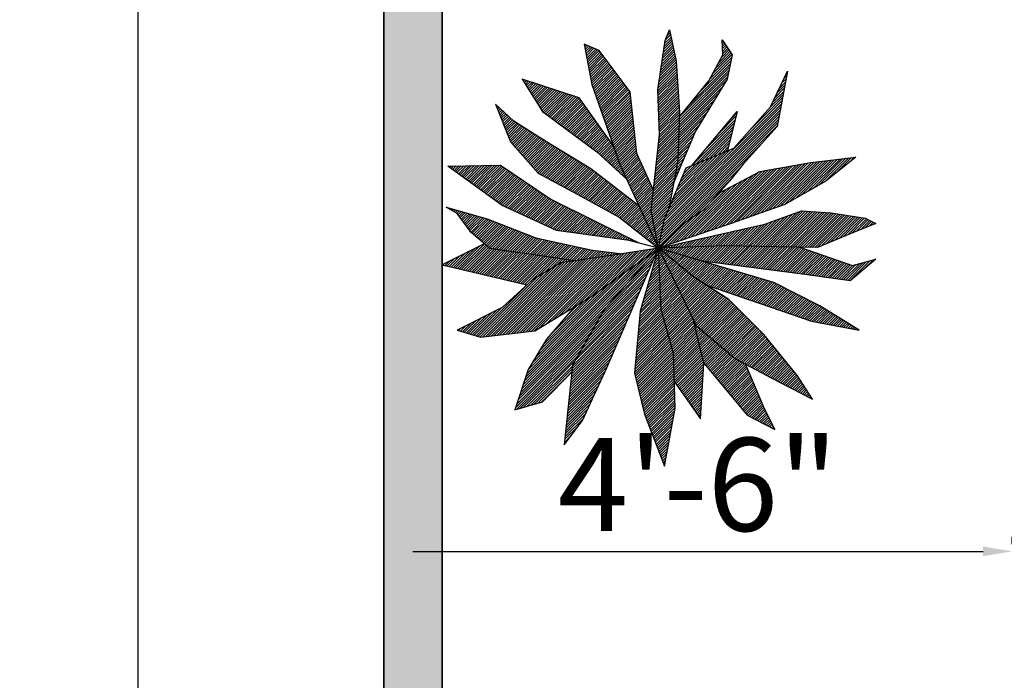
# Model space of a CAD drawing. Units: inches. Extents: x 3008 to 4088, y 1255 to 2137.
# Tile 11 of 30: x 3008 to 3093, y 1787 to 1844. Entities that reach past the tile are written whole.
import ezdxf

# ---------------------------------------------------------------- set-up
doc = ezdxf.new("R2010")
doc.units = ezdxf.units.IN
for name, color, linetype, lineweight in [('A-ANNO-DIMS', 2, 'Continuous', 18), ('C-PROP', 1, 'Continuous', 35), ('C-PROP-PATT', 9, 'Continuous', 13), ('L-PLNT', 3, 'Continuous', 13), ('vfolhas', 114, 'Continuous', 5)]:
    doc.layers.add(name, color=color, linetype=linetype, lineweight=lineweight)
for name, color, linetype in [('vfolha', 72, 'Continuous'), ('vfolha2', 110, 'Continuous'), ('vfolhas2', 102, 'Continuous')]:
    doc.layers.add(name, color=color, linetype=linetype)
doc.styles.get("Standard").update_dxf_attribs({"font": 'arial.ttf'})
doc.dimstyles.new('ISO-25', dxfattribs={"dimtxt": 8, "dimasz": 2.5, "dimexe": 1.25, "dimexo": 0.625, "dimtad": 1, "dimdec": 1, "dimlunit": 3, "dimtxsty": 'Standard', "dimcen": 2.5, "dimadec": 0, "dimazin": 0, "dimtfac": 1, "dimtdec": 1, "dimtmove": 0, "dimatfit": 3, "dimfxl": 1, "dimarcsym": 0})
pattern_1 = [(45, (-2446.5133113, 50.986076), (-0.004419417382, 0.004419417382), [])]

# ---------------------------------------------------------------- blocks, each defined once
blk = doc.blocks.new('*D2')
at = {"layer": 'A-ANNO-DIMS', "color": 0, "lineweight": -2, "transparency": 16777216}
for p, q in [((3039.041, 2003.966), (3017.26, 2003.966)), ((3018.51, 2001.466), (3018.51, 1346.466)), ((3039.041, 1343.966), (3017.26, 1343.966))]:
    blk.add_line(p, q, dxfattribs=at)
at = {"layer": 'A-ANNO-DIMS', "color": 0, "transparency": 16777216}
for points in [[(3018.093, 2001.466), (3018.927, 2001.466), (3018.51, 2003.966)], [(3018.093, 1346.466), (3018.927, 1346.466), (3018.51, 1343.966)]]:
    blk.add_solid(points, dxfattribs=at)
at = {"layer": 'Defpoints', "color": 0, "transparency": 16777216}
for p in [(3039.666, 2003.966), (3018.51, 1343.966), (3039.666, 1343.966)]:
    blk.add_point(p, dxfattribs=at)
at = {"layer": 'A-ANNO-DIMS', "color": 0, "transparency": 16777216, "insert": (3013.817, 1673.966), "char_height": 8, "attachment_point": 5, "rotation": 90}
blk.add_mtext("55'", dxfattribs=at)
blk = doc.blocks.new('*D3')
at = {"layer": 'A-ANNO-DIMS', "color": 0, "lineweight": -2, "transparency": 16777216}
for p, q in [((3039.666, 1798.574), (3039.666, 1799.199)), ((3093.666, 1798.574), (3093.666, 1799.199)), ((3042.166, 1797.949), (3091.166, 1797.949))]:
    blk.add_line(p, q, dxfattribs=at)
at = {"layer": 'A-ANNO-DIMS', "color": 0, "transparency": 16777216}
for points in [[(3042.166, 1798.366), (3042.166, 1797.532), (3039.666, 1797.949)], [(3091.166, 1798.366), (3091.166, 1797.532), (3093.666, 1797.949)]]:
    blk.add_solid(points, dxfattribs=at)
at = {"layer": 'Defpoints', "color": 0, "transparency": 16777216}
for p in [(3039.666, 1797.949), (3093.666, 1797.949), (3093.666, 1797.949)]:
    blk.add_point(p, dxfattribs=at)
at = {"layer": 'A-ANNO-DIMS', "color": 0, "transparency": 16777216, "insert": (3066.666, 1802.659), "char_height": 8, "attachment_point": 5}
blk.add_mtext('4\'-6"', dxfattribs=at)
blk = doc.blocks.new('arbusto_PB_verde_grande')
at = {"layer": 'vfolha2'}
h = blk.add_hatch(dxfattribs=at)
h.set_pattern_fill('ANSI31', color=256, scale=0.05, style=0)
h.set_pattern_definition(pattern_1)
h.paths.add_polyline_path([(0.0294, 0.3565), (0.0003, 0.0905), (0.0263, -0.0393), (0.047, 0.0623), (0.0619, 0.0973), (0.0937, 0.2657), (0.0996, 0.4347), (0.0879, 0.6131), (0.0645, 0.7227), (0.0499, 0.6851), (0.0236, 0.5129)])
h.paths.add_polyline_path([(0.3011, 0.4379), (0.1423, 0.2487), (0.2669, 0.3002)])
h.paths.add_polyline_path([(0.38, 0.2282), (0.237, 0.1519), (0.1843, 0.0936), (0.1112, 0.0436), (0.0263, -0.0393), (0.2806, 0.0467), (0.3683, 0.078), (0.4676, 0.1124), (0.6107, 0.1938), (0.7159, 0.2782), (0.5581, 0.2595)])
h.paths.add_polyline_path([(0.561, -0.2944), (0.7275, -0.3257), (0.5902, -0.2412), (0.4296, -0.1598), (0.0263, -0.0393), (0.1492, -0.1411), (0.1884, -0.166), (0.415, -0.2444)])
h.paths.add_polyline_path([(-0.2743, -0.4478), (-0.3035, -0.7263), (-0.2392, -0.6417), (-0.1546, -0.4572), (0.0263, -0.0393), (-0.1633, -0.2538)])
h.paths.add_polyline_path([(-0.5196, -0.2474), (-0.6774, -0.3257), (-0.5956, -0.3507), (-0.4057, -0.3288), (-0.2101, -0.21), (0.0263, -0.0393), (-0.1487, -0.0659), (-0.3152, -0.091), (-0.4145, -0.1505)])
h.paths.add_polyline_path([(-0.5255, 0.2501), (-0.7095, 0.247), (-0.5196, 0.1093), (-0.3298, 0.0217), (-0.0757, -0.0128), (-0.0423, -0.0215), (-0.3502, 0.1312)])
h = blk.add_hatch(dxfattribs=at)
h.set_pattern_fill('ANSI31', color=256, scale=0.05, style=0)
h.set_pattern_definition(pattern_1)
h.paths.add_polyline_path([(-0.1896, 0.297), (-0.0855, 0.2019), (-0.1078, 0.2501), (-0.132, 0.3187), (-0.251, 0.4848), (-0.4495, 0.5505), (-0.3795, 0.4379)])
h.paths.add_polyline_path([(0.0791, -0.4071), (0.0821, -0.5063), (0.1726, -0.6355), (0.1843, -0.4415), (0.149, -0.2918), (0.0263, -0.0393), (0.0353, -0.2538)])
at = {"layer": 'vfolhas'}
h = blk.add_hatch(dxfattribs=at)
h.set_pattern_fill('ANSI31', color=256, scale=0.05, style=0)
h.set_pattern_definition(pattern_1)
h.paths.add_polyline_path([(-0.0728, 0.5067), (-0.1808, 0.6506), (-0.2334, 0.6725), (-0.2071, 0.5318), (-0.1078, 0.2501), (0.0263, -0.0393), (0.0003, 0.0905), (0.0082, 0.1624), (-0.0494, 0.2908)])
h.paths.add_polyline_path([(0.099, 0.4193), (0.0937, 0.2657), (0.0791, 0.1881), (0.1551, 0.369), (0.2661, 0.5505), (0.2836, 0.635), (0.2485, 0.6882), (0.2514, 0.635), (0.2018, 0.5443)])
h.paths.add_polyline_path([(0.1229, 0.2407), (0.047, 0.0623), (0.0263, -0.0393), (0.1112, 0.0436), (0.1843, 0.0936), (0.2748, 0.1938), (0.3215, 0.2532), (0.4413, 0.3847), (0.4763, 0.5787), (0.4179, 0.4535), (0.2894, 0.3095)])
h.paths.add_polyline_path([(0.5815, -0.0378), (0.7071, 0.0154), (0.7859, 0.0467), (0.748, 0.0655), (0.6282, 0.0842), (0.526, 0.0905), (0.3974, 0.0436), (0.0263, -0.0393), (0.2573, -0.0315), (0.4383, -0.0347)])
h.paths.add_polyline_path([(0.5202, -0.0365), (0.4383, -0.0347), (0.2573, -0.0315), (0.0263, -0.0393), (0.1796, -0.0852), (0.5377, -0.1317), (0.6954, -0.1536), (0.7859, -0.0785), (0.7041, -0.1004)])
h.paths.add_polyline_path([(0.2719, -0.2193), (0.1492, -0.1411), (0.0263, -0.0393), (0.1579, -0.3101), (0.2952, -0.4258), (0.4179, -0.4916), (0.564, -0.5667), (0.5114, -0.4853), (0.3946, -0.3414)])
h.paths.add_polyline_path([(-0.0582, -0.4759), (-0.0231, -0.6198), (0.047, -0.8013), (0.0849, -0.5979), (0.0791, -0.4071), (0.0353, -0.2538), (0.0263, -0.0393), (-0.0377, -0.26)])
h.paths.add_polyline_path([(-0.2422, 0.1405), (-0.1107, 0.0686), (0.0263, -0.0393), (-0.0423, 0.1087), (-0.2101, 0.2376), (-0.3649, 0.3314), (-0.4787, 0.4034), (-0.543, 0.4629), (-0.4904, 0.3314), (-0.3941, 0.2219)])
h = blk.add_hatch(dxfattribs=at)
h.set_pattern_fill('ANSI31', color=256, scale=0.05, style=0)
h.set_pattern_definition(pattern_1)
h.paths.add_polyline_path([(-0.5722, 0.0623), (-0.7153, 0.103), (-0.6774, 0.0811), (-0.6277, 0.0154), (-0.5635, -0.041), (-0.2646, -0.0834), (-0.1487, -0.0659), (-0.1015, -0.0588), (-0.2042, -0.0472), (-0.4028, -0.0034)])
h.paths.add_polyline_path([(-0.5635, -0.041), (-0.5828, -0.024), (-0.7299, -0.0973), (-0.4334, -0.1679), (-0.4145, -0.1505), (-0.3152, -0.091), (-0.2646, -0.0834)])
h.paths.add_polyline_path([(-0.2769, -0.4727), (-0.2743, -0.4478), (-0.1633, -0.2538), (0.0263, -0.0393), (-0.2101, -0.21), (-0.2672, -0.2447), (-0.3649, -0.357), (-0.4291, -0.4634), (-0.4759, -0.6043), (-0.3795, -0.576)])
h = blk.add_hatch(dxfattribs=at)
h.set_pattern_fill('ANSI31', color=256, scale=0.05, style=0)
h.set_pattern_definition(pattern_1)
h.paths.add_polyline_path([(0.3361, -0.623), (0.4325, -0.6731), (0.3946, -0.5948), (0.3303, -0.4446), (0.2952, -0.4258), (0.1579, -0.3101), (0.149, -0.2918), (0.1843, -0.4415)])
at = {"layer": 'vfolha'}
for p, q in [((0.0263, -0.0393), (-0.1487, -0.0659)), ((0.0263, -0.0393), (-0.0377, -0.26)), ((0.0353, -0.2538), (0.0263, -0.0393)), ((0.5202, -0.0365), (0.7041, -0.1004)), ((0.5377, -0.1317), (0.1796, -0.0852)), ((0.7859, -0.0785), (0.6954, -0.1536)), ((0.7041, -0.1004), (0.7859, -0.0785)), ((0.6954, -0.1536), (0.5377, -0.1317)), ((0.3946, -0.3414), (0.2719, -0.2193)), ((-0.2672, -0.2447), (-0.3649, -0.357)), ((-0.0377, -0.26), (-0.0582, -0.4759)), ((0.0791, -0.4071), (0.0353, -0.2538)), ((0.1579, -0.3101), (0.2952, -0.4258)), ((0.5114, -0.4853), (0.3946, -0.3414)), ((0.0849, -0.5979), (0.0791, -0.4071)), ((0.2952, -0.4258), (0.4179, -0.4916)), ((0.4179, -0.4916), (0.564, -0.5667)), ((0.564, -0.5667), (0.5114, -0.4853)), ((0.047, -0.8013), (0.0849, -0.5979)), ((-0.0231, -0.6198), (0.047, -0.8013))]:
    blk.add_line(p, q, dxfattribs=at)
at = {"layer": 'vfolha2'}
for p, q in [((0.0499, 0.6851), (0.0645, 0.7227)), ((0.0645, 0.7227), (0.0879, 0.6131)), ((0.0236, 0.5129), (0.0499, 0.6851)), ((0.0879, 0.6131), (0.0996, 0.4347)), ((-0.4495, 0.5505), (-0.3795, 0.4379)), ((-0.251, 0.4848), (-0.4495, 0.5505)), ((-0.132, 0.3187), (-0.251, 0.4848)), ((0.0294, 0.3565), (0.0236, 0.5129)), ((-0.3795, 0.4379), (-0.1896, 0.297)), ((0.0996, 0.4347), (0.0937, 0.2657)), ((0.1434, 0.2501), (0.3011, 0.4379)), ((0.3011, 0.4379), (0.2661, 0.297)), ((0.0003, 0.0905), (0.0294, 0.3565)), ((-0.1896, 0.297), (-0.0822, 0.1989)), ((0.5581, 0.2595), (0.7159, 0.2782)), ((0.7159, 0.2782), (0.6107, 0.1938)), ((-0.7095, 0.247), (-0.5255, 0.2501)), ((-0.5196, 0.1093), (-0.7095, 0.247)), ((-0.5255, 0.2501), (-0.3502, 0.1312)), ((0.38, 0.2282), (0.5581, 0.2595)), ((0.237, 0.1519), (0.38, 0.2282)), ((0.6107, 0.1938), (0.4676, 0.1124)), ((-0.3298, 0.0217), (-0.5196, 0.1093)), ((-0.3502, 0.1312), (-0.0423, -0.0215)), ((0.0263, -0.0393), (0.0003, 0.0905)), ((0.3683, 0.078), (0.2806, 0.0467)), ((0.2806, 0.0467), (0.0263, -0.0393)), ((-0.0757, -0.0128), (-0.3298, 0.0217)), ((-0.1487, -0.0659), (-0.3152, -0.091)), ((-0.2101, -0.21), (0.0263, -0.0393)), ((0.0263, -0.0393), (-0.1633, -0.2538)), ((-0.1546, -0.4572), (0.0263, -0.0393)), ((0.4296, -0.1598), (0.0263, -0.0393)), ((0.0263, -0.0393), (0.1579, -0.3101)), ((-0.3152, -0.091), (-0.4145, -0.1505)), ((-0.4145, -0.1505), (-0.5196, -0.2474)), ((0.1884, -0.166), (0.415, -0.2444)), ((0.5902, -0.2412), (0.4296, -0.1598)), ((-0.4057, -0.3288), (-0.2101, -0.21)), ((-0.5196, -0.2474), (-0.6774, -0.3257)), ((-0.1633, -0.2538), (-0.2743, -0.4478)), ((0.415, -0.2444), (0.561, -0.2944)), ((0.7275, -0.3257), (0.5902, -0.2412)), ((0.1843, -0.4415), (0.149, -0.2918)), ((0.561, -0.2944), (0.7275, -0.3257)), ((-0.6774, -0.3257), (-0.5956, -0.3507)), ((-0.5956, -0.3507), (-0.4057, -0.3288)), ((0.1726, -0.6355), (0.1843, -0.4415)), ((-0.2743, -0.4478), (-0.3035, -0.7263)), ((0.0821, -0.5063), (0.1726, -0.6355)), ((-0.3035, -0.7263), (-0.2392, -0.6417))]:
    blk.add_line(p, q, dxfattribs=at)
at = {"layer": 'vfolhas2'}
for p, q in [((0.2514, 0.635), (0.2485, 0.6882)), ((0.2485, 0.6882), (0.2836, 0.635)), ((-0.2334, 0.6725), (-0.2071, 0.5318)), ((-0.1808, 0.6506), (-0.2334, 0.6725)), ((-0.0728, 0.5067), (-0.1808, 0.6506)), ((0.2018, 0.5443), (0.2514, 0.635)), ((0.2836, 0.635), (0.2661, 0.5505)), ((0.2661, 0.5505), (0.1551, 0.369)), ((0.4179, 0.4535), (0.4763, 0.5787)), ((0.4763, 0.5787), (0.4413, 0.3847)), ((-0.2071, 0.5318), (-0.1078, 0.2501)), ((0.099, 0.4193), (0.2018, 0.5443)), ((-0.0494, 0.2908), (-0.0728, 0.5067)), ((-0.543, 0.4629), (-0.4904, 0.3314)), ((-0.4787, 0.4034), (-0.543, 0.4629)), ((0.2894, 0.3095), (0.4179, 0.4535)), ((-0.3649, 0.3314), (-0.4787, 0.4034)), ((0.4413, 0.3847), (0.3215, 0.2532)), ((0.1551, 0.369), (0.078, 0.1855)), ((-0.4904, 0.3314), (-0.3941, 0.2219)), ((-0.2101, 0.2376), (-0.3649, 0.3314)), ((0.0082, 0.1624), (-0.0494, 0.2908)), ((0.1229, 0.2407), (0.2894, 0.3095)), ((-0.1078, 0.2501), (0.0263, -0.0393)), ((0.0937, 0.2657), (0.0619, 0.0973)), ((0.3215, 0.2532), (0.2748, 0.1938)), ((-0.3941, 0.2219), (-0.2422, 0.1405)), ((-0.0423, 0.1087), (-0.2101, 0.2376)), ((0.047, 0.0623), (0.1229, 0.2407)), ((0.2748, 0.1938), (0.1843, 0.0936)), ((-0.2422, 0.1405), (-0.1107, 0.0686)), ((0.4676, 0.1124), (0.3683, 0.078)), ((-0.6774, 0.0811), (-0.7153, 0.103)), ((-0.7153, 0.103), (-0.5722, 0.0623)), ((-0.6277, 0.0154), (-0.6774, 0.0811)), ((0.1843, 0.0936), (0.1112, 0.0436)), ((0.3974, 0.0436), (0.526, 0.0905)), ((0.526, 0.0905), (0.6282, 0.0842)), ((0.6282, 0.0842), (0.748, 0.0655)), ((-0.5722, 0.0623), (-0.4028, -0.0034)), ((-0.1107, 0.0686), (0.0263, -0.0393)), ((0.0263, -0.0393), (0.047, 0.0623)), ((0.0263, -0.0393), (0.3974, 0.0436)), ((0.1112, 0.0436), (0.0263, -0.0393)), ((0.7859, 0.0467), (0.7071, 0.0154)), ((0.748, 0.0655), (0.7859, 0.0467)), ((-0.5635, -0.041), (-0.6277, 0.0154)), ((0.7071, 0.0154), (0.5815, -0.0378)), ((-0.5828, -0.024), (-0.7299, -0.0973)), ((-0.4028, -0.0034), (-0.2042, -0.0472)), ((0.0263, -0.0393), (-0.0757, -0.0128)), ((0.2573, -0.0315), (0.0263, -0.0393)), ((0.4383, -0.0347), (0.2573, -0.0315)), ((-0.2646, -0.0834), (-0.5635, -0.041)), ((-0.2042, -0.0472), (-0.0983, -0.0591)), ((0.1492, -0.1411), (0.0263, -0.0393)), ((0.5815, -0.0378), (0.4383, -0.0347)), ((-0.7299, -0.0973), (-0.4334, -0.1679)), ((0.2719, -0.2193), (0.1492, -0.1411)), ((-0.3649, -0.357), (-0.4291, -0.4634)), ((0.1843, -0.4415), (0.3361, -0.623)), ((0.3946, -0.5948), (0.329, -0.4417)), ((-0.4291, -0.4634), (-0.4759, -0.6043)), ((-0.3795, -0.576), (-0.2769, -0.4727)), ((-0.2392, -0.6417), (-0.1546, -0.4572)), ((-0.0582, -0.4759), (-0.0231, -0.6198)), ((-0.4759, -0.6043), (-0.3795, -0.576)), ((0.4325, -0.6731), (0.3946, -0.5948)), ((0.3361, -0.623), (0.4325, -0.6731))]:
    blk.add_line(p, q, dxfattribs=at)

msp = doc.modelspace()

# ---------------------------------------------------------------- hatches: boundary and pattern name
at = {"layer": 'C-PROP-PATT'}
h = msp.add_hatch(color=256, dxfattribs=at)
h.dxf.hatch_style = 1
h.paths.add_polyline_path([(3519.666, 2003.966), (3039.666, 2003.966), (3039.666, 1343.966), (3051.666, 1343.966), (3051.666, 1348.966), (3044.666, 1348.966), (3044.666, 1998.966), (3514.666, 1998.966), (3514.666, 1348.966), (3219.666, 1348.966), (3219.666, 1343.966), (3519.666, 1343.966)])

# ---------------------------------------------------------------- linework, layer by layer
at = {"layer": 'C-PROP'}
for p, q in [((3039.666, 1343.966), (3039.666, 2003.966)), ((3044.666, 1348.966), (3044.666, 1998.966))]:
    msp.add_line(p, q, dxfattribs=at)

# ---------------------------------------------------------------- block references
at = {"layer": 'L-PLNT', "xscale": 24.60366729364114, "yscale": 24.60366729364114, "zscale": 24.60366729364114}
msp.add_blockref('arbusto_PB_verde_grande', (3062.624, 1824.969), dxfattribs=at)

# ---------------------------------------------------------------- dimensions: what is measured, and where the dimension line sits
at = {"layer": 'A-ANNO-DIMS'}
dim = msp.add_linear_dim(base=(3018.51, 1343.966), p1=(3039.666, 2003.966), p2=(3039.666, 1343.966), angle=90, dimstyle='ISO-25', override={"dimclrd": 0, "dimclre": 0, "dimclrt": 0}, dxfattribs=at)
dim.commit()
dim.dimension.update_dxf_attribs({"geometry": '*D2', "text_midpoint": (3013.817, 1673.966)})
dim = msp.add_linear_dim(base=(3093.666, 1797.949), p1=(3039.666, 1797.949), p2=(3093.666, 1797.949), dimstyle='ISO-25', override={"dimclrd": 0, "dimclre": 0, "dimclrt": 0}, dxfattribs=at)
dim.commit()
dim.dimension.update_dxf_attribs({"geometry": '*D3', "text_midpoint": (3066.666, 1802.659)})

doc.saveas('drawing.dxf')
